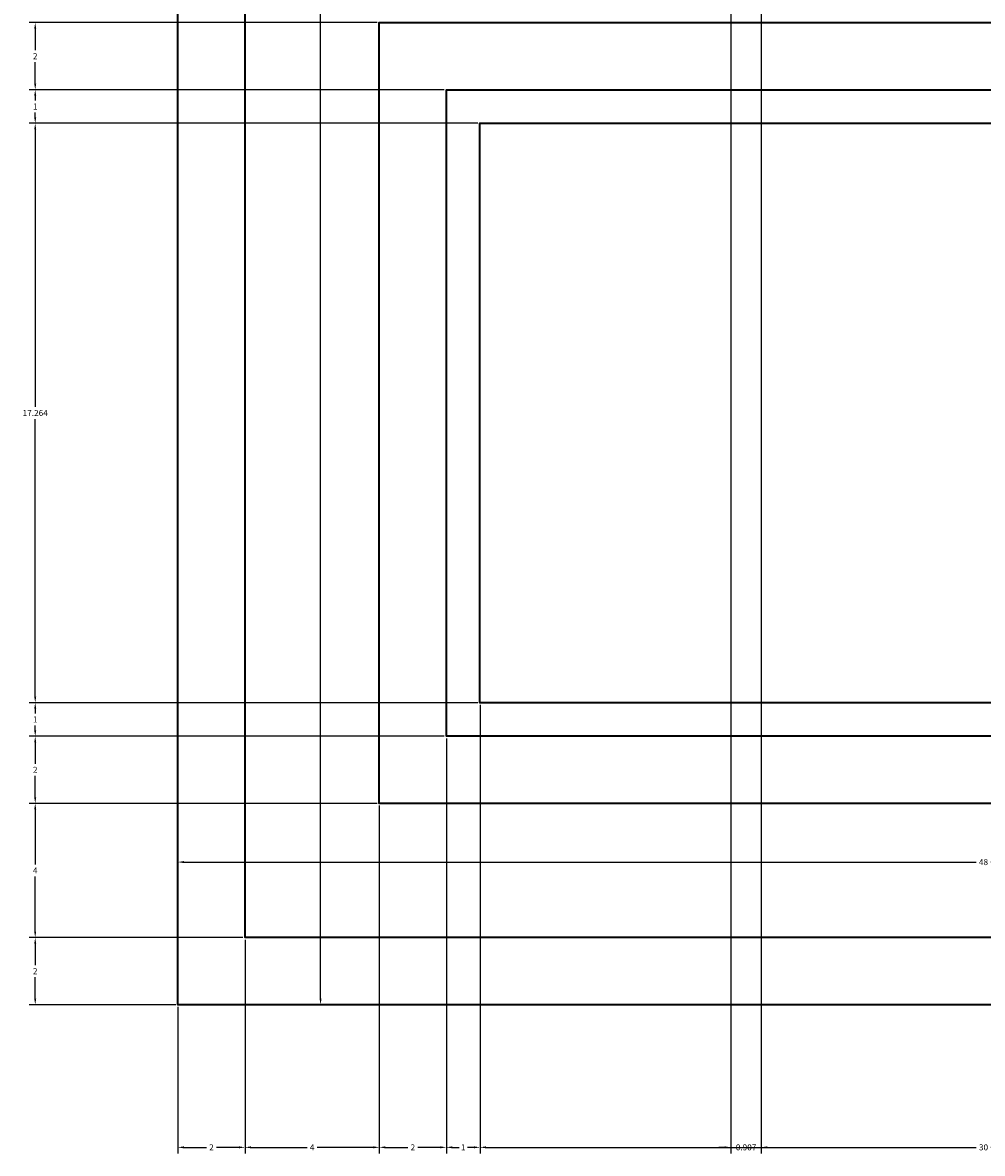
# Model space of a CAD drawing. Units: inches. Extents: x 3137 to 3299, y 1994 to 2089.
# Tile 1 of 14: x 3137 to 3165, y 1994 to 2028. Entities that reach past the tile are written whole.
import ezdxf

# ---------------------------------------------------------------- set-up
doc = ezdxf.new("R2010")
doc.units = ezdxf.units.IN
doc.header["$MEASUREMENT"] = 0
for name, color, linetype, lineweight in [('A-ANNO-DIMS', 2, 'Continuous', 18), ('A-ANNO-NPLT', 8, 'Continuous', 13), ('A-DOOR', 4, 'Continuous', 35)]:
    doc.layers.add(name, color=color, linetype=linetype, lineweight=lineweight)
doc.styles.get("Standard").update_dxf_attribs({"font": 'arial.ttf'})
doc.dimstyles.get("Standard").update_dxf_attribs({"dimtxt": 0.18, "dimasz": 0.18, "dimexe": 0.18, "dimexo": 0.0625, "dimgap": 0.09, "dimtad": 0, "dimtih": 1, "dimtoh": 1, "dimdec": 4, "dimzin": 0, "dimdsep": 46, "dimtxsty": 'Standard', "dimcen": 0.09, "dimadec": 0, "dimazin": 0, "dimtfac": 1, "dimtdec": 4, "dimtofl": 0, "dimtmove": 0, "dimatfit": 3, "dimfxl": 1, "dimtolj": 1, "dimtzin": 0, "dimarcsym": 0})

# ---------------------------------------------------------------- blocks, each defined once
blk = doc.blocks.new('*D13')
at = {"layer": 'A-ANNO-DIMS', "color": 0, "lineweight": -2, "transparency": 16777216}
for p, q in [((3141.478, 1998.936), (3141.478, 2003.304)), ((3141.658, 2003.124), (3165.255, 2003.124)), ((3189.298, 2003.124), (3165.7, 2003.124)), ((3189.478, 1998.936), (3189.478, 2003.304))]:
    blk.add_line(p, q, dxfattribs=at)
at = {"layer": 'A-ANNO-DIMS', "color": 0, "transparency": 16777216}
for points in [[(3141.658, 2003.154), (3141.658, 2003.094), (3141.478, 2003.124)], [(3189.298, 2003.154), (3189.298, 2003.094), (3189.478, 2003.124)]]:
    blk.add_solid(points, dxfattribs=at)
at = {"layer": 'Defpoints', "color": 0, "transparency": 16777216}
for p in [(3189.478, 2003.124), (3141.478, 1998.874), (3189.478, 1998.874)]:
    blk.add_point(p, dxfattribs=at)
at = {"layer": 'A-ANNO-DIMS', "color": 0, "transparency": 16777216, "insert": (3165.478, 2003.124), "char_height": 0.18, "attachment_point": 5}
blk.add_mtext('\\A1;48', dxfattribs=at)
blk = doc.blocks.new('*D14')
at = {"layer": 'A-ANNO-DIMS', "color": 0, "lineweight": -2, "transparency": 16777216}
for p, q in [((3143.478, 2000.811), (3143.478, 1994.444)), ((3141.478, 1998.811), (3141.478, 1994.444)), ((3141.658, 1994.624), (3142.328, 1994.624)), ((3143.298, 1994.624), (3142.627, 1994.624))]:
    blk.add_line(p, q, dxfattribs=at)
at = {"layer": 'A-ANNO-DIMS', "color": 0, "transparency": 16777216}
for points in [[(3141.658, 1994.654), (3141.658, 1994.594), (3141.478, 1994.624)], [(3143.298, 1994.654), (3143.298, 1994.594), (3143.478, 1994.624)]]:
    blk.add_solid(points, dxfattribs=at)
at = {"layer": 'Defpoints', "color": 0, "transparency": 16777216}
for p in [(3143.478, 2000.874), (3141.478, 1998.874), (3143.478, 1994.624)]:
    blk.add_point(p, dxfattribs=at)
at = {"layer": 'A-ANNO-DIMS', "color": 0, "transparency": 16777216, "insert": (3142.478, 1994.624), "char_height": 0.18, "attachment_point": 5}
blk.add_mtext('\\A1;2', dxfattribs=at)
blk = doc.blocks.new('*D15')
at = {"layer": 'A-ANNO-DIMS', "color": 0, "lineweight": -2, "transparency": 16777216}
for p, q in [((3147.478, 2004.811), (3147.478, 1994.444)), ((3143.478, 2000.811), (3143.478, 1994.444)), ((3143.658, 1994.624), (3145.325, 1994.624)), ((3147.298, 1994.624), (3145.63, 1994.624))]:
    blk.add_line(p, q, dxfattribs=at)
at = {"layer": 'A-ANNO-DIMS', "color": 0, "transparency": 16777216}
for points in [[(3143.658, 1994.654), (3143.658, 1994.594), (3143.478, 1994.624)], [(3147.298, 1994.654), (3147.298, 1994.594), (3147.478, 1994.624)]]:
    blk.add_solid(points, dxfattribs=at)
at = {"layer": 'Defpoints', "color": 0, "transparency": 16777216}
for p in [(3147.478, 2004.874), (3143.478, 2000.874), (3147.478, 1994.624)]:
    blk.add_point(p, dxfattribs=at)
at = {"layer": 'A-ANNO-DIMS', "color": 0, "transparency": 16777216, "insert": (3145.478, 1994.624), "char_height": 0.18, "attachment_point": 5}
blk.add_mtext('\\A1;4', dxfattribs=at)
blk = doc.blocks.new('*D16')
at = {"layer": 'A-ANNO-DIMS', "color": 0, "lineweight": -2, "transparency": 16777216}
for p, q in [((3149.478, 2006.811), (3149.478, 1994.444)), ((3147.478, 2004.811), (3147.478, 1994.444)), ((3147.658, 1994.624), (3148.328, 1994.624)), ((3149.298, 1994.624), (3148.627, 1994.624))]:
    blk.add_line(p, q, dxfattribs=at)
at = {"layer": 'A-ANNO-DIMS', "color": 0, "transparency": 16777216}
for points in [[(3147.658, 1994.654), (3147.658, 1994.594), (3147.478, 1994.624)], [(3149.298, 1994.654), (3149.298, 1994.594), (3149.478, 1994.624)]]:
    blk.add_solid(points, dxfattribs=at)
at = {"layer": 'Defpoints', "color": 0, "transparency": 16777216}
for p in [(3149.478, 2006.874), (3147.478, 2004.874), (3149.478, 1994.624)]:
    blk.add_point(p, dxfattribs=at)
at = {"layer": 'A-ANNO-DIMS', "color": 0, "transparency": 16777216, "insert": (3148.478, 1994.624), "char_height": 0.18, "attachment_point": 5}
blk.add_mtext('\\A1;2', dxfattribs=at)
blk = doc.blocks.new('*D17')
at = {"layer": 'A-ANNO-DIMS', "color": 0, "lineweight": -2, "transparency": 16777216}
for p, q in [((3150.478, 2007.811), (3150.478, 1994.444)), ((3149.478, 2006.811), (3149.478, 1994.444)), ((3149.658, 1994.624), (3149.855, 1994.624)), ((3150.298, 1994.624), (3150.101, 1994.624))]:
    blk.add_line(p, q, dxfattribs=at)
at = {"layer": 'A-ANNO-DIMS', "color": 0, "transparency": 16777216}
for points in [[(3149.658, 1994.654), (3149.658, 1994.594), (3149.478, 1994.624)], [(3150.298, 1994.654), (3150.298, 1994.594), (3150.478, 1994.624)]]:
    blk.add_solid(points, dxfattribs=at)
at = {"layer": 'Defpoints', "color": 0, "transparency": 16777216}
for p in [(3150.478, 2007.874), (3149.478, 2006.874), (3150.478, 1994.624)]:
    blk.add_point(p, dxfattribs=at)
at = {"layer": 'A-ANNO-DIMS', "color": 0, "transparency": 16777216, "insert": (3149.978, 1994.624), "char_height": 0.18, "attachment_point": 5}
blk.add_mtext('\\A1;1', dxfattribs=at)
blk = doc.blocks.new('*D18')
at = {"layer": 'A-ANNO-DIMS', "color": 0, "lineweight": -2, "transparency": 16777216}
for p, q in [((3150.478, 2007.811), (3150.478, 1994.444)), ((3180.478, 2007.811), (3180.478, 1994.444)), ((3150.658, 1994.624), (3165.259, 1994.624)), ((3180.298, 1994.624), (3165.696, 1994.624))]:
    blk.add_line(p, q, dxfattribs=at)
at = {"layer": 'A-ANNO-DIMS', "color": 0, "transparency": 16777216}
for points in [[(3150.658, 1994.654), (3150.658, 1994.594), (3150.478, 1994.624)], [(3180.298, 1994.654), (3180.298, 1994.594), (3180.478, 1994.624)]]:
    blk.add_solid(points, dxfattribs=at)
at = {"layer": 'Defpoints', "color": 0, "transparency": 16777216}
for p in [(3150.478, 2007.874), (3180.478, 2007.874), (3180.478, 1994.624)]:
    blk.add_point(p, dxfattribs=at)
at = {"layer": 'A-ANNO-DIMS', "color": 0, "transparency": 16777216, "insert": (3165.478, 1994.624), "char_height": 0.18, "attachment_point": 5}
blk.add_mtext('\\A1;30', dxfattribs=at)
blk = doc.blocks.new('*D34')
at = {"layer": 'A-ANNO-DIMS', "color": 0, "lineweight": -2, "transparency": 16777216}
for p, q in [((3143.415, 2000.874), (3137.048, 2000.874)), ((3137.228, 2000.694), (3137.228, 2000.054)), ((3137.228, 1999.054), (3137.228, 1999.694)), ((3141.415, 1998.874), (3137.048, 1998.874))]:
    blk.add_line(p, q, dxfattribs=at)
at = {"layer": 'A-ANNO-DIMS', "color": 0, "transparency": 16777216}
for points in [[(3137.198, 2000.694), (3137.258, 2000.694), (3137.228, 2000.874)], [(3137.198, 1999.054), (3137.258, 1999.054), (3137.228, 1998.874)]]:
    blk.add_solid(points, dxfattribs=at)
at = {"layer": 'Defpoints', "color": 0, "transparency": 16777216}
for p in [(3137.228, 2000.874), (3143.478, 2000.874), (3141.478, 1998.874)]:
    blk.add_point(p, dxfattribs=at)
at = {"layer": 'A-ANNO-DIMS', "color": 0, "transparency": 16777216, "insert": (3137.228, 1999.874), "char_height": 0.18, "attachment_point": 5}
blk.add_mtext('\\A1;2', dxfattribs=at)
blk = doc.blocks.new('*D35')
at = {"layer": 'A-ANNO-DIMS', "color": 0, "lineweight": -2, "transparency": 16777216}
for p, q in [((3147.415181, 2004.873967), (3137.047681, 2004.873967)), ((3137.227681, 2004.693967), (3137.227681, 2003.053967)), ((3137.227681, 2001.053967), (3137.227681, 2002.693967)), ((3143.415181, 2000.873967), (3137.047681, 2000.873967))]:
    blk.add_line(p, q, dxfattribs=at)
at = {"layer": 'A-ANNO-DIMS', "color": 0, "transparency": 16777216}
for points in [[(3137.197681, 2004.693967), (3137.257681, 2004.693967), (3137.227681, 2004.873967)], [(3137.197681, 2001.053967), (3137.257681, 2001.053967), (3137.227681, 2000.873967)]]:
    blk.add_solid(points, dxfattribs=at)
at = {"layer": 'Defpoints', "color": 0, "transparency": 16777216}
for p in [(3137.227681, 2004.873967), (3147.477681, 2004.873967), (3143.477681, 2000.873967)]:
    blk.add_point(p, dxfattribs=at)
at = {"layer": 'A-ANNO-DIMS', "color": 0, "transparency": 16777216, "insert": (3137.227681, 2002.873967), "char_height": 0.18, "attachment_point": 5}
blk.add_mtext('\\A1;4', dxfattribs=at)
blk = doc.blocks.new('*D36')
at = {"layer": 'A-ANNO-DIMS', "color": 0, "lineweight": -2, "transparency": 16777216}
for p, q in [((3149.415, 2006.874), (3137.048, 2006.874)), ((3137.228, 2006.694), (3137.228, 2006.054)), ((3137.228, 2005.054), (3137.228, 2005.694)), ((3147.415, 2004.874), (3137.048, 2004.874))]:
    blk.add_line(p, q, dxfattribs=at)
at = {"layer": 'A-ANNO-DIMS', "color": 0, "transparency": 16777216}
for points in [[(3137.198, 2006.694), (3137.258, 2006.694), (3137.228, 2006.874)], [(3137.198, 2005.054), (3137.258, 2005.054), (3137.228, 2004.874)]]:
    blk.add_solid(points, dxfattribs=at)
at = {"layer": 'Defpoints', "color": 0, "transparency": 16777216}
for p in [(3137.228, 2006.874), (3149.478, 2006.874), (3147.478, 2004.874)]:
    blk.add_point(p, dxfattribs=at)
at = {"layer": 'A-ANNO-DIMS', "color": 0, "transparency": 16777216, "insert": (3137.228, 2005.874), "char_height": 0.18, "attachment_point": 5}
blk.add_mtext('\\A1;2', dxfattribs=at)
blk = doc.blocks.new('*D37')
at = {"layer": 'A-ANNO-DIMS', "color": 0, "lineweight": -2, "transparency": 16777216}
for p, q in [((3150.415, 2007.874), (3137.048, 2007.874)), ((3137.228, 2007.694), (3137.228, 2007.554)), ((3137.228, 2007.054), (3137.228, 2007.194)), ((3149.415, 2006.874), (3137.048, 2006.874))]:
    blk.add_line(p, q, dxfattribs=at)
at = {"layer": 'A-ANNO-DIMS', "color": 0, "transparency": 16777216}
for points in [[(3137.198, 2007.694), (3137.258, 2007.694), (3137.228, 2007.874)], [(3137.198, 2007.054), (3137.258, 2007.054), (3137.228, 2006.874)]]:
    blk.add_solid(points, dxfattribs=at)
at = {"layer": 'Defpoints', "color": 0, "transparency": 16777216}
for p in [(3137.228, 2007.874), (3150.478, 2007.874), (3149.478, 2006.874)]:
    blk.add_point(p, dxfattribs=at)
at = {"layer": 'A-ANNO-DIMS', "color": 0, "transparency": 16777216, "insert": (3137.228, 2007.374), "char_height": 0.18, "attachment_point": 5}
blk.add_mtext('\\A1;1', dxfattribs=at)
blk = doc.blocks.new('*D38')
at = {"layer": 'A-ANNO-DIMS', "color": 0, "lineweight": -2, "transparency": 16777216}
for p, q in [((3150.415, 2025.138), (3137.048, 2025.138)), ((3137.228, 2024.958), (3137.228, 2016.688)), ((3137.228, 2008.054), (3137.228, 2016.324)), ((3150.415, 2007.874), (3137.048, 2007.874))]:
    blk.add_line(p, q, dxfattribs=at)
at = {"layer": 'A-ANNO-DIMS', "color": 0, "transparency": 16777216}
for points in [[(3137.198, 2024.958), (3137.258, 2024.958), (3137.228, 2025.138)], [(3137.198, 2008.054), (3137.258, 2008.054), (3137.228, 2007.874)]]:
    blk.add_solid(points, dxfattribs=at)
at = {"layer": 'Defpoints', "color": 0, "transparency": 16777216}
for p in [(3137.228, 2025.138), (3150.478, 2025.138), (3150.478, 2007.874)]:
    blk.add_point(p, dxfattribs=at)
at = {"layer": 'A-ANNO-DIMS', "color": 0, "transparency": 16777216, "insert": (3137.228, 2016.506), "char_height": 0.18, "attachment_point": 5}
blk.add_mtext('\\A1;17.264', dxfattribs=at)
blk = doc.blocks.new('*D39')
at = {"layer": 'A-ANNO-DIMS', "color": 0, "lineweight": -2, "transparency": 16777216}
for p, q in [((3149.415, 2026.138), (3137.048, 2026.138)), ((3137.228, 2025.958), (3137.228, 2025.818)), ((3137.228, 2025.318), (3137.228, 2025.457)), ((3150.415, 2025.138), (3137.048, 2025.138))]:
    blk.add_line(p, q, dxfattribs=at)
at = {"layer": 'A-ANNO-DIMS', "color": 0, "transparency": 16777216}
for points in [[(3137.198, 2025.958), (3137.258, 2025.958), (3137.228, 2026.138)], [(3137.198, 2025.318), (3137.258, 2025.318), (3137.228, 2025.138)]]:
    blk.add_solid(points, dxfattribs=at)
at = {"layer": 'Defpoints', "color": 0, "transparency": 16777216}
for p in [(3137.228, 2026.138), (3149.478, 2026.138), (3150.478, 2025.138)]:
    blk.add_point(p, dxfattribs=at)
at = {"layer": 'A-ANNO-DIMS', "color": 0, "transparency": 16777216, "insert": (3137.228, 2025.638), "char_height": 0.18, "attachment_point": 5}
blk.add_mtext('\\A1;1', dxfattribs=at)
blk = doc.blocks.new('*D40')
at = {"layer": 'A-ANNO-DIMS', "color": 0, "lineweight": -2, "transparency": 16777216}
for p, q in [((3147.415, 2028.138), (3137.048, 2028.138)), ((3137.228, 2027.958), (3137.228, 2027.318)), ((3137.228, 2026.318), (3137.228, 2026.957)), ((3149.415, 2026.138), (3137.048, 2026.138))]:
    blk.add_line(p, q, dxfattribs=at)
at = {"layer": 'A-ANNO-DIMS', "color": 0, "transparency": 16777216}
for points in [[(3137.198, 2027.958), (3137.258, 2027.958), (3137.228, 2028.138)], [(3137.198, 2026.318), (3137.258, 2026.318), (3137.228, 2026.138)]]:
    blk.add_solid(points, dxfattribs=at)
at = {"layer": 'Defpoints', "color": 0, "transparency": 16777216}
for p in [(3137.228, 2028.138), (3147.478, 2028.138), (3149.478, 2026.138)]:
    blk.add_point(p, dxfattribs=at)
at = {"layer": 'A-ANNO-DIMS', "color": 0, "transparency": 16777216, "insert": (3137.228, 2027.138), "char_height": 0.18, "attachment_point": 5}
blk.add_mtext('\\A1;2', dxfattribs=at)
blk = doc.blocks.new('*D55')
at = {"layer": 'A-ANNO-DIMS', "color": 0, "lineweight": -2, "transparency": 16777216}
for p, q in [((3141.54, 2082.874), (3145.908, 2082.874)), ((3145.728, 2082.694), (3145.728, 2041.056)), ((3145.728, 1999.054), (3145.728, 2040.692)), ((3141.54, 1998.874), (3145.908, 1998.874))]:
    blk.add_line(p, q, dxfattribs=at)
at = {"layer": 'A-ANNO-DIMS', "color": 0, "transparency": 16777216}
for points in [[(3145.698, 2082.694), (3145.758, 2082.694), (3145.728, 2082.874)], [(3145.698, 1999.054), (3145.758, 1999.054), (3145.728, 1998.874)]]:
    blk.add_solid(points, dxfattribs=at)
at = {"layer": 'Defpoints', "color": 0, "transparency": 16777216}
for p in [(3141.478, 2082.874), (3141.478, 1998.874), (3145.728, 1998.874)]:
    blk.add_point(p, dxfattribs=at)
at = {"layer": 'A-ANNO-DIMS', "color": 0, "transparency": 16777216, "insert": (3145.728, 2040.874), "char_height": 0.18, "attachment_point": 5}
blk.add_mtext('\\A1;84', dxfattribs=at)
blk = doc.blocks.new('*D81')
at = {"layer": 'A-ANNO-DIMS', "color": 0, "lineweight": -2, "transparency": 16777216}
for p, q in [((3157.951, 2066.849), (3157.951, 1994.444)), ((3158.858, 2065.44), (3158.858, 1994.444)), ((3157.771, 1994.624), (3157.591, 1994.624)), ((3159.038, 1994.624), (3159.218, 1994.624))]:
    blk.add_line(p, q, dxfattribs=at)
at = {"layer": 'A-ANNO-DIMS', "color": 0, "transparency": 16777216}
for points in [[(3157.771, 1994.654), (3157.771, 1994.594), (3157.951, 1994.624)], [(3159.038, 1994.654), (3159.038, 1994.594), (3158.858, 1994.624)]]:
    blk.add_solid(points, dxfattribs=at)
at = {"layer": 'Defpoints', "color": 0, "transparency": 16777216}
for p in [(3157.951, 2066.911), (3158.858, 2065.503), (3158.858, 1994.624)]:
    blk.add_point(p, dxfattribs=at)
at = {"layer": 'A-ANNO-DIMS', "color": 0, "transparency": 16777216, "insert": (3158.404, 1994.624), "char_height": 0.18, "attachment_point": 5}
blk.add_mtext('\\A1;0.907', dxfattribs=at)

msp = doc.modelspace()

# ---------------------------------------------------------------- linework, layer by layer
at = {"layer": 'A-ANNO-NPLT'}
msp.add_point((3147.4777, 2004.874), dxfattribs=at)
at = {"layer": 'A-DOOR'}
for points in [[(3141.4777, 2082.874), (3189.4777, 2082.874), (3189.4777, 1998.874), (3141.4777, 1998.874)], [(3183.4777, 2028.1375), (3183.4777, 2004.874), (3147.4777, 2004.874), (3147.4777, 2028.1375)], [(3181.4777, 2026.1375), (3181.4777, 2006.874), (3149.4777, 2006.874), (3149.4777, 2026.1375)], [(3180.4777, 2025.1375), (3180.4777, 2007.874), (3150.4777, 2007.874), (3150.4777, 2025.1375)]]:
    msp.add_lwpolyline(points, close=True, dxfattribs=at)
msp.add_lwpolyline([(3187.4777, 2007.6773), (3187.4777, 2000.874), (3143.4777, 2000.874), (3143.4777, 2080.874), (3187.4777, 2080.874), (3187.4777, 2076.298)], dxfattribs=at)

# ---------------------------------------------------------------- dimensions: what is measured, and where the dimension line sits
at = {"layer": 'A-ANNO-DIMS'}
for base, p1, p2, angle, override, picture, middle in [((3145.7277, 1998.874), (3141.4777, 2082.874), (3141.4777, 1998.874), 270, {"dimdec": 0, "dimlfac": 1, "dimrnd": 0, "dimzin": 0, "dimdsep": 46, "dimlunit": 2}, '*D55', (3145.7277, 2040.874)), ((3137.2277, 2028.1375), (3149.4777, 2026.1375), (3147.4777, 2028.1375), 90, {"dimdec": 0, "dimlfac": 1, "dimrnd": 0, "dimzin": 0, "dimdsep": 46, "dimlunit": 2}, '*D40', (3137.2277, 2027.1375)), ((3137.2277, 2026.1375), (3150.4777, 2025.1375), (3149.4777, 2026.1375), 90, {"dimdec": 0, "dimlfac": 1, "dimrnd": 0, "dimzin": 0, "dimdsep": 46, "dimlunit": 2}, '*D39', (3137.2277, 2025.6375)), ((3137.22768, 2025.13754), (3150.47768, 2007.87397), (3150.47768, 2025.13754), 90, {"dimdec": 3, "dimlfac": 1, "dimrnd": 0, "dimzin": 0, "dimdsep": 46, "dimlunit": 2}, '*D38', (3137.22768, 2016.50575)), ((3137.2277, 2007.874), (3149.4777, 2006.874), (3150.4777, 2007.874), 90, {"dimdec": 0, "dimlfac": 1, "dimrnd": 0, "dimzin": 0, "dimdsep": 46, "dimlunit": 2}, '*D37', (3137.2277, 2007.374)), ((3137.2277, 2006.874), (3147.4777, 2004.874), (3149.4777, 2006.874), 90, {"dimdec": 0, "dimlfac": 1, "dimrnd": 0, "dimzin": 0, "dimdsep": 46, "dimlunit": 2}, '*D36', (3137.2277, 2005.874)), ((3137.2277, 2004.874), (3143.4777, 2000.874), (3147.4777, 2004.874), 90, {"dimdec": 0, "dimlfac": 1, "dimrnd": 0, "dimzin": 0, "dimdsep": 46, "dimlunit": 2}, '*D35', (3137.2277, 2002.874)), ((3137.2277, 2000.874), (3141.4777, 1998.874), (3143.4777, 2000.874), 90, {"dimdec": 0, "dimlfac": 1, "dimrnd": 0, "dimzin": 0, "dimdsep": 46, "dimlunit": 2}, '*D34', (3137.2277, 1999.874))]:
    dim = msp.add_linear_dim(base=base, p1=p1, p2=p2, angle=angle, dimstyle='Standard', override=override, dxfattribs=at)
    dim.commit()
    dim.dimension.update_dxf_attribs({"geometry": picture, "text_midpoint": middle})
for base, p1, p2, override, picture, middle in [((3158.8577, 1994.624), (3157.9507, 2066.9111), (3158.8577, 2065.5029), {"dimdec": 3, "dimlfac": 1, "dimrnd": 0, "dimzin": 0, "dimdsep": 46, "dimlunit": 2}, '*D81', (3158.4042, 1994.624)), ((3150.4777, 1994.624), (3149.4777, 2006.874), (3150.4777, 2007.874), {"dimdec": 0, "dimlfac": 1, "dimrnd": 0, "dimzin": 0, "dimdsep": 46, "dimlunit": 2}, '*D17', (3149.9777, 1994.624)), ((3180.4777, 1994.624), (3150.4777, 2007.874), (3180.4777, 2007.874), {"dimdec": 0, "dimlfac": 1, "dimrnd": 0, "dimzin": 0, "dimdsep": 46, "dimlunit": 2}, '*D18', (3165.4777, 1994.624)), ((3149.4777, 1994.624), (3147.4777, 2004.874), (3149.4777, 2006.874), {"dimdec": 0, "dimlfac": 1, "dimrnd": 0, "dimzin": 0, "dimdsep": 46, "dimlunit": 2}, '*D16', (3148.4777, 1994.624)), ((3147.4777, 1994.624), (3143.4777, 2000.874), (3147.4777, 2004.874), {"dimdec": 0, "dimlfac": 1, "dimrnd": 0, "dimzin": 0, "dimdsep": 46, "dimlunit": 2}, '*D15', (3145.4777, 1994.624)), ((3189.4777, 2003.124), (3141.4777, 1998.874), (3189.4777, 1998.874), {"dimdec": 0, "dimlfac": 1, "dimrnd": 0, "dimzin": 0, "dimdsep": 46, "dimlunit": 2}, '*D13', (3165.4777, 2003.124)), ((3143.4777, 1994.624), (3141.4777, 1998.874), (3143.4777, 2000.874), {"dimdec": 0, "dimlfac": 1, "dimrnd": 0, "dimzin": 0, "dimdsep": 46, "dimlunit": 2}, '*D14', (3142.4777, 1994.624))]:
    dim = msp.add_linear_dim(base=base, p1=p1, p2=p2, dimstyle='Standard', override=override, dxfattribs=at)
    dim.commit()
    dim.dimension.update_dxf_attribs({"geometry": picture, "text_midpoint": middle})

doc.saveas('drawing.dxf')
